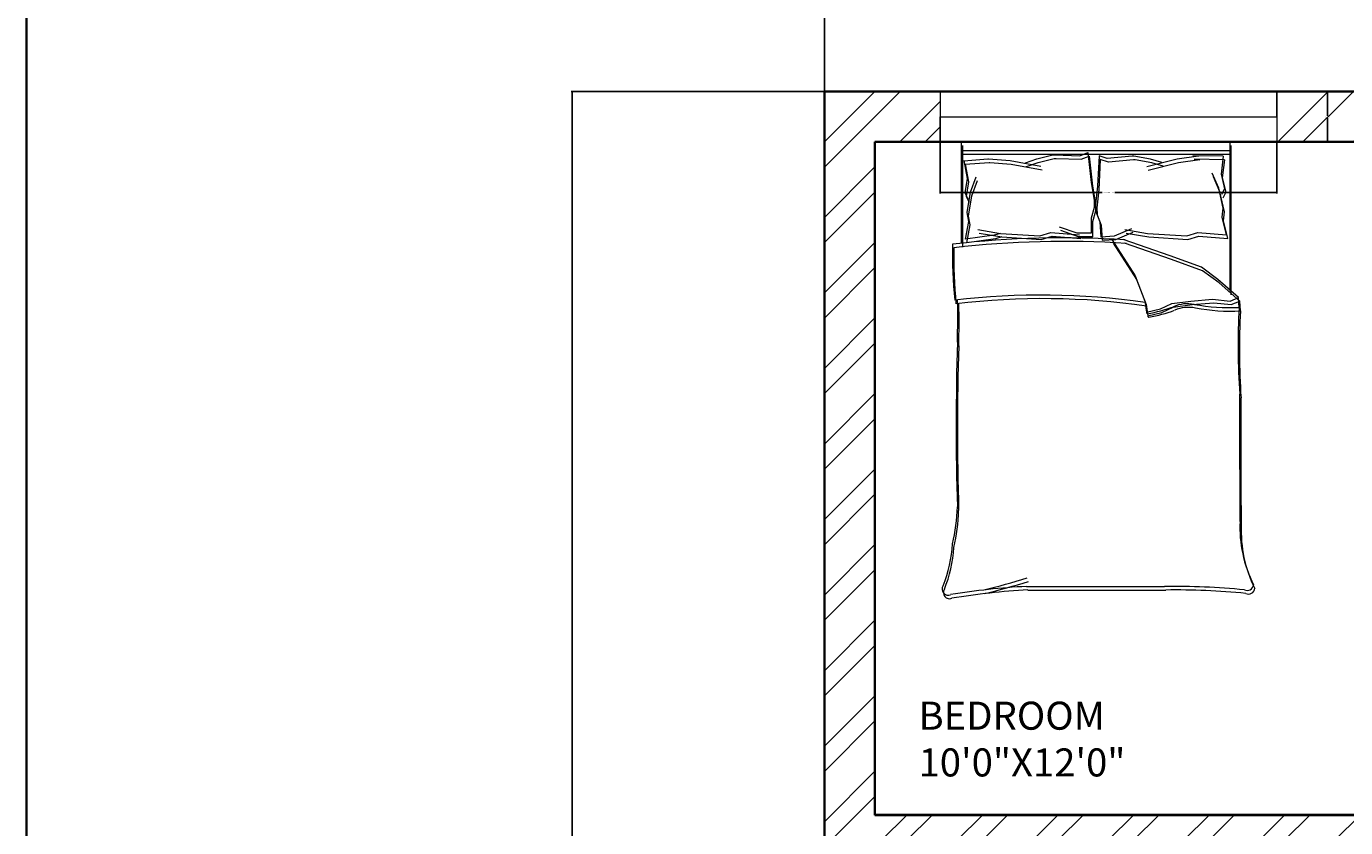
# Model space of a CAD drawing. Units: inches. Extents: x 2120 to 4013, y 1390 to 3019.
# Tile 29 of 59: x 2120 to 2356, y 2221 to 2364. Entities that reach past the tile are written whole.
import ezdxf

# ---------------------------------------------------------------- set-up
doc = ezdxf.new("R2010")
doc.units = ezdxf.units.IN
for name, color, linetype, lineweight in [('A-ANNO-DIMS', 2, 'Continuous', 18), ('A-ANNO-TTLB', 7, 'Continuous', 35), ('A-AREA-IDEN', 7, 'Continuous', 18), ('A-FURN', 8, 'Continuous', 13), ('A-GLAZ', 4, 'Continuous', 18), ('A-WALL', 7, 'Continuous', 35), ('A-WALL-PATT', 252, 'Continuous', 13)]:
    doc.layers.add(name, color=color, linetype=linetype, lineweight=lineweight)
doc.styles.get("Standard").update_dxf_attribs({"font": 'arial.ttf'})
doc.dimstyles.get("Standard").update_dxf_attribs({"dimtxt": 0.18, "dimasz": 0.18, "dimexe": 0.18, "dimexo": 0.0625, "dimgap": 0.09, "dimtad": 0, "dimtih": 1, "dimtoh": 1, "dimdec": 4, "dimzin": 0, "dimdsep": 46, "dimtxsty": 'Standard', "dimcen": 0.09, "dimadec": 0, "dimazin": 0, "dimtfac": 1, "dimtdec": 4, "dimtofl": 0, "dimtmove": 0, "dimatfit": 3, "dimfxl": 1, "dimtolj": 1, "dimtzin": 0, "dimarcsym": 0})

# ---------------------------------------------------------------- blocks, each defined once
blk = doc.blocks.new('BED-DOUBLE-PLAN')
for p, q in [((3.48, 63.34), (3.48, 81.45)), ((3.48, 81.45), (51.27, 81.45)), ((3.7, 62.7), (3.7, 80.81)), ((51.27, 81.45), (51.27, 54.84)), ((51.5, 80.81), (51.5, 54.2)), ((3.48, 79.91), (51.27, 79.91)), ((3.7, 79.27), (51.5, 79.27)), ((3.9, 78.11), (8.18, 78.44)), ((3.9, 78.13), (4.47, 74.95)), ((4.13, 77.47), (8.41, 77.8)), ((8.18, 78.44), (8.29, 78.42)), ((8.29, 78.42), (12.11, 78.13)), ((8.41, 77.8), (8.51, 77.78)), ((8.51, 77.78), (12.34, 77.49)), ((12.11, 78.13), (17.6, 77.12)), ((14.86, 77.7), (16.88, 78.42)), ((15.08, 77.06), (17.11, 77.78)), ((16.88, 78.42), (19.77, 79.14)), ((17.11, 77.78), (20, 78.5)), ((19.77, 79.14), (20.09, 79.14)), ((20, 78.5), (20.32, 78.5)), ((20.09, 79.14), (24.54, 79)), ((20.32, 78.5), (24.77, 78.36)), ((24.54, 79), (25.98, 79.58)), ((24.77, 78.36), (26.21, 78.94)), ((25.98, 79.58), (26.56, 74.23)), ((26.21, 78.94), (26.79, 73.59)), ((27.98, 78.95), (27.73, 73.58)), ((28.21, 78.32), (27.96, 72.94)), ((29.46, 78.47), (27.98, 78.95)), ((29.69, 77.83), (28.21, 78.32)), ((33.89, 78.89), (29.46, 78.47)), ((34.11, 78.25), (29.69, 77.83)), ((34.21, 78.91), (33.89, 78.89)), ((34.43, 78.27), (34.11, 78.25)), ((37.14, 78.37), (34.21, 78.91)), ((37.37, 77.73), (34.43, 78.27)), ((41.92, 78.38), (36.5, 77.02)), ((42.14, 77.74), (36.72, 76.38)), ((39.2, 77.77), (37.14, 78.37)), ((39.43, 77.13), (37.37, 77.73)), ((45.71, 78.9), (41.92, 78.38)), ((45.94, 78.26), (42.14, 77.74)), ((50.11, 78.89), (44.71, 78.99)), ((44.71, 78.99), (45.71, 78.9)), ((50.34, 78.25), (44.94, 78.35)), ((44.94, 78.35), (45.94, 78.26)), ((50.11, 78.89), (49.73, 75.68)), ((50.34, 78.25), (49.96, 75.04)), ((4.12, 77.49), (4.7, 74.31)), ((12.34, 77.49), (17.83, 76.48)), ((49.31, 73.19), (48.13, 75.87)), ((49.73, 75.68), (50.33, 73.11)), ((4.47, 74.95), (4.04, 72.35)), ((4.7, 74.31), (4.27, 71.71)), ((5.05, 72.49), (6.06, 75.24)), ((5.28, 71.85), (6.29, 74.6)), ((26.56, 74.23), (27.14, 71.05)), ((26.79, 73.59), (27.37, 70.41)), ((27.73, 73.58), (27.36, 70.37)), ((27.96, 72.94), (27.58, 69.73)), ((49.54, 72.55), (48.36, 75.23)), ((50.11, 69.62), (49.31, 73.19)), ((50.33, 73.11), (49.82, 72.06)), ((49.96, 75.04), (50.56, 72.47)), ((4.04, 72.35), (4.62, 71.33)), ((4.27, 71.71), (4.85, 70.7)), ((4.47, 68.88), (5.05, 72.49)), ((4.7, 68.24), (5.28, 71.85)), ((27.14, 71.05), (27.14, 69.74)), ((50.34, 68.98), (49.54, 72.55)), ((50.56, 72.47), (50.04, 71.42)), ((4.76, 67.29), (4.47, 68.88)), ((4.99, 66.65), (4.7, 68.24)), ((27.14, 69.74), (26.56, 67.86)), ((27.37, 69.1), (26.79, 67.23)), ((27.36, 70.37), (27.44, 69.07)), ((27.37, 70.41), (27.37, 69.1)), ((27.44, 69.07), (28.13, 67.23)), ((27.58, 69.73), (27.67, 68.43)), ((27.67, 68.43), (28.36, 66.59)), ((49.92, 68.01), (50.11, 69.62)), ((50.15, 67.37), (50.34, 68.98)), ((4.19, 64.11), (4.76, 67.29)), ((4.41, 63.47), (4.99, 66.65)), ((24.1, 65.18), (20.96, 66.27)), ((26.56, 67.86), (26.56, 65.18)), ((26.79, 67.23), (26.79, 64.54)), ((28.13, 67.23), (28.3, 64.55)), ((28.36, 66.59), (28.53, 63.91)), ((30.75, 64.71), (33.82, 65.99)), ((50.7, 64.87), (49.92, 68.01)), ((50.93, 64.23), (50.15, 67.37)), ((9.28, 64.83), (4.19, 64.11)), ((9.51, 64.19), (4.41, 63.47)), ((6.38, 65.82), (10.42, 65.15)), ((6.61, 65.18), (10.64, 64.51)), ((10.42, 65.15), (9.28, 64.83)), ((10.64, 64.51), (9.51, 64.19)), ((10.42, 65.15), (17.43, 64.72)), ((10.64, 64.51), (17.65, 64.08)), ((17.43, 64.72), (19.39, 65.28)), ((17.65, 64.08), (19.61, 64.64)), ((19.39, 65.28), (24.52, 64.87)), ((19.61, 64.64), (24.75, 64.23)), ((24.33, 64.54), (21.19, 65.63)), ((26.56, 65.18), (24.1, 65.18)), ((26.79, 64.54), (24.33, 64.54)), ((28.3, 64.55), (30.75, 64.71)), ((28.53, 63.91), (30.98, 64.07)), ((30.26, 64.06), (34.45, 57.57)), ((30.98, 64.07), (34.05, 65.35)), ((40.65, 61.13), (32.31, 64.06)), ((32.57, 65.82), (36.6, 65.15)), ((32.79, 65.18), (36.83, 64.51)), ((36.6, 65.15), (43.61, 64.72)), ((36.83, 64.51), (43.84, 64.08)), ((43.61, 64.72), (45.57, 65.28)), ((43.84, 64.08), (45.8, 64.64)), ((45.57, 65.28), (50.7, 64.87)), ((45.8, 64.64), (50.93, 64.23)), ((30.49, 63.42), (34.68, 56.93)), ((40.87, 60.49), (32.54, 63.42)), ((46.22, 59.12), (40.65, 61.13)), ((46.45, 58.48), (40.87, 60.49)), ((49.16, 56.95), (46.22, 59.12)), ((34.45, 57.57), (36.15, 53.08)), ((34.68, 56.93), (36.38, 52.44)), ((49.39, 56.31), (46.45, 58.48)), ((52.87, 53.7), (49.16, 56.95)), ((53.1, 53.06), (49.39, 56.31)), ((36.15, 53.08), (36.46, 51.07)), ((36.38, 52.44), (36.69, 50.43)), ((38.94, 51.69), (40.96, 52.62)), ((39.17, 51.05), (41.18, 51.98)), ((40.96, 52.62), (44.36, 53.08)), ((41.18, 51.98), (44.59, 52.44)), ((44.36, 53.08), (48.23, 53.39)), ((44.59, 52.44), (48.46, 52.75)), ((48.23, 53.39), (51.33, 53.08)), ((48.46, 52.75), (51.56, 52.44)), ((51.33, 53.08), (52.87, 53.7)), ((51.56, 52.44), (53.1, 53.06)), ((52.95, 51.96), (52.87, 53.7, 3.87)), ((53.18, 51.32), (53.1, 53.06, 3.87)), ((36.46, 51.07), (38.94, 51.69)), ((36.69, 50.43), (39.17, 51.05)), ((15.06, 2.2), (39.68, 2.2)), ((15.29, 1.56), (39.91, 1.56))]:
    blk.add_line(p, q)
for centre, radius, start, end in [((21.36, -100.61), 164.97, 86.0865, 96.7821), ((21.59, -101.25), 164.97, 86.0865, 96.7821), ((85.16, 61.35), 83.31, 178.7218, 185.604), ((85.39, 60.71), 83.31, 178.7218, 185.604), ((17.76, -74.87), 129.02, 81.7845, 96.9006), ((17.99, -75.51), 129.02, 81.7845, 96.9006), ((-167.31, 50.27), 170.11, 358.4762, 1.0082), ((-167.08, 49.63), 170.11, 358.4762, 1.0082), ((31.16, 79.96), 29.65, 280.6617, 289.8806), ((43.74, 46.38), 6.22, 78.6608, 113.7384), ((43.97, 45.74), 6.22, 78.6608, 113.7384), ((51.33, 88.1), 36.18, 259.8763, 272.5657), ((51.56, 87.46), 36.18, 259.8763, 272.5657), ((182.27, 45.13), 129.5, 176.9791, 183.8365), ((36.64, 51.01), 0.185, 160.2464, 271.1377), ((36.87, 50.37), 0.185, 160.2464, 271.1377), ((31.38, 79.32), 29.65, 280.6617, 289.8806), ((182.5, 44.49), 129.5, 176.9791, 183.8365), ((484.82, 30.83), 482.31, 178.2277, 181.7185), ((485.05, 30.19), 482.31, 178.2277, 181.7185), ((-4508.74, 13.62), 4561.86, 0.00217, 0.28689), ((-4508.51, 12.99), 4561.86, 0.00217, 0.28689), ((-26.9, 16.93), 29.63, 346.0648, 358.9113), ((-26.67, 16.29), 29.63, 346.0648, 358.9113), ((76.16, 12.78), 23.07, 177.4714, 206.4681), ((76.39, 12.14), 23.07, 177.4714, 206.4681), ((-21.66, 11.17), 23.56, 337.9751, 356.652), ((-21.43, 10.53), 23.56, 337.9751, 356.652), ((-17.22, 105.16), 106.46, 283.3832, 287.7053), ((-16.99, 104.52), 106.46, 283.3832, 287.7053), ((54.41, 2.58), 1.1, 242.6588, 356.02), ((1.09, 1.73), 1.09, 146.1736, 293.4781), ((1.32, 1.09), 1.09, 146.1736, 293.4781), ((21.43, -119.39), 121.76, 92.9958, 99.4091), ((21.66, -120.03), 121.76, 92.9958, 99.4091), ((41.15, -130.83), 133.04, 84.4998, 90.6351), ((41.38, -131.47), 133.04, 84.4998, 90.6351), ((54.64, 1.94), 1.1, 242.6588, 356.02)]:
    blk.add_arc(centre, radius, start, end)
blk = doc.blocks.new('WIN-PLAN-60IN')
for p, q in [((0, 9), (0, 0)), ((60, 4.5), (60, 9)), ((60, 9), (60, 0)), ((0, 0), (0, 4.5)), ((0, 4.5), (60, 4.5))]:
    blk.add_line(p, q)
blk = doc.blocks.new('*D171')
at = {"layer": 'A-ANNO-DIMS', "color": 0, "lineweight": -2, "transparency": 16777216}
for p, q in [((2283.38, 2343.47), (2283.38, 2334.35)), ((2343.38, 2343.47), (2343.38, 2334.35)), ((2283.56, 2334.53), (2312.26, 2334.53)), ((2343.2, 2334.53), (2314.5, 2334.53))]:
    blk.add_line(p, q, dxfattribs=at)
at = {"layer": 'A-ANNO-DIMS', "color": 0, "transparency": 16777216}
for points in [[(2283.56, 2334.56), (2283.56, 2334.5), (2283.38, 2334.53)], [(2343.2, 2334.56), (2343.2, 2334.5), (2343.38, 2334.53)]]:
    blk.add_solid(points, dxfattribs=at)
at = {"layer": 'Defpoints', "color": 0, "transparency": 16777216}
for p in [(2283.38, 2343.53), (2343.38, 2343.53), (2343.38, 2334.53)]:
    blk.add_point(p, dxfattribs=at)
at = {"layer": 'A-ANNO-DIMS', "color": 0, "transparency": 16777216, "insert": (2313.38, 2334.53), "char_height": 0.18, "attachment_point": 5}
blk.add_mtext('\\A1;WINDOW 60 TYP.', dxfattribs=at)
blk = doc.blocks.new('*D172')
at = {"layer": 'A-ANNO-DIMS', "color": 0, "lineweight": -2, "transparency": 16777216}
for p, q in [((2343.44, 2352.53), (2352.56, 2352.53)), ((2352.38, 2352.35), (2352.38, 2348.21)), ((2352.38, 2343.71), (2352.38, 2347.85)), ((2343.44, 2343.53), (2352.56, 2343.53))]:
    blk.add_line(p, q, dxfattribs=at)
at = {"layer": 'A-ANNO-DIMS', "color": 0, "transparency": 16777216}
for points in [[(2352.35, 2352.35), (2352.41, 2352.35), (2352.38, 2352.53)], [(2352.35, 2343.71), (2352.41, 2343.71), (2352.38, 2343.53)]]:
    blk.add_solid(points, dxfattribs=at)
at = {"layer": 'Defpoints', "color": 0, "transparency": 16777216}
for p in [(2343.38, 2352.53), (2352.38, 2352.53), (2343.38, 2343.53)]:
    blk.add_point(p, dxfattribs=at)
at = {"layer": 'A-ANNO-DIMS', "color": 0, "transparency": 16777216, "insert": (2352.38, 2348.03), "char_height": 0.18, "attachment_point": 5}
blk.add_mtext('\\A1;9 TYP.', dxfattribs=at)
blk = doc.blocks.new('*D211')
at = {"layer": 'A-ANNO-DIMS', "color": 0, "lineweight": -2, "transparency": 16777216}
for p, q in [((2262.73, 2352.59), (2262.73, 2397.71)), ((2262.91, 2397.53), (2635.95, 2397.53)), ((3009.55, 2397.53), (2636.52, 2397.53)), ((3009.73, 2352.59), (3009.73, 2397.71))]:
    blk.add_line(p, q, dxfattribs=at)
at = {"layer": 'A-ANNO-DIMS', "color": 0, "transparency": 16777216}
for points in [[(2262.91, 2397.56), (2262.91, 2397.5), (2262.73, 2397.53)], [(3009.55, 2397.56), (3009.55, 2397.5), (3009.73, 2397.53)]]:
    blk.add_solid(points, dxfattribs=at)
at = {"layer": 'Defpoints', "color": 0, "transparency": 16777216}
for p in [(3009.73, 2397.53), (2262.73, 2352.53), (3009.73, 2352.53)]:
    blk.add_point(p, dxfattribs=at)
at = {"layer": 'A-ANNO-DIMS', "color": 0, "transparency": 16777216, "insert": (2636.23, 2397.53), "char_height": 0.18, "attachment_point": 5}
blk.add_mtext('\\A1;747', dxfattribs=at)
blk = doc.blocks.new('*D215')
at = {"layer": 'A-ANNO-DIMS', "color": 0, "lineweight": -2, "transparency": 16777216}
for p, q in [((2262.67, 2352.53), (2217.55, 2352.53)), ((2217.73, 2352.35), (2217.73, 2213.96)), ((2217.73, 2075.21), (2217.73, 2213.6)), ((2271.67, 2075.03), (2217.55, 2075.03))]:
    blk.add_line(p, q, dxfattribs=at)
at = {"layer": 'A-ANNO-DIMS', "color": 0, "transparency": 16777216}
for points in [[(2217.7, 2352.35), (2217.76, 2352.35), (2217.73, 2352.53)], [(2217.7, 2075.21), (2217.76, 2075.21), (2217.73, 2075.03)]]:
    blk.add_solid(points, dxfattribs=at)
at = {"layer": 'Defpoints', "color": 0, "transparency": 16777216}
for p in [(2217.73, 2352.53), (2262.73, 2352.53), (2271.73, 2075.03)]:
    blk.add_point(p, dxfattribs=at)
at = {"layer": 'A-ANNO-DIMS', "color": 0, "transparency": 16777216, "insert": (2217.73, 2213.78), "char_height": 0.18, "attachment_point": 5}
blk.add_mtext('\\A1;277.5', dxfattribs=at)

msp = doc.modelspace()

# ---------------------------------------------------------------- hatches: boundary and pattern name
at = {"layer": 'A-WALL-PATT'}
h = msp.add_hatch(dxfattribs=at)
h.set_pattern_fill('ANSI32', color=256)
h.paths.add_polyline_path([(2271.7331, 2343.531), (2283.3788, 2343.531), (2283.3788, 2348.031), (2283.3788, 2352.5306), (2262.7331, 2352.5306), (2262.7331, 2182.638), (2267.2331, 2182.638), (2271.7331, 2182.638), (2271.7331, 2219.031), (2391.7331, 2219.031), (2391.7331, 2214.189), (2393.9831, 2214.189), (2396.2331, 2214.189), (2396.2331, 2219.031), (2420.2331, 2219.031), (2420.2331, 2225.7535), (2417.2197, 2225.7535), (2415.7331, 2225.7535), (2415.7331, 2223.5306), (2271.7331, 2223.5306)])
h.paths.add_polyline_path([(2380.0942, 2352.5306), (2343.3788, 2352.5306), (2343.3788, 2343.531), (2363.2331, 2343.531), (2363.2331, 2288.8489), (2365.4831, 2288.8489), (2367.7331, 2288.8489), (2367.7331, 2343.531), (2380.0942, 2343.531)], flags=17)
h.paths.add_polyline_path([(2432.4339, 2352.5306), (2404.0943, 2352.5306), (2404.0943, 2343.531), (2415.7331, 2343.531), (2415.7331, 2264.0306), (2367.7331, 2264.0306), (2367.7331, 2266.4872), (2363.2331, 2266.4872), (2363.2331, 2259.531), (2367.7331, 2259.531), (2415.7331, 2259.531), (2415.7331, 2255.0658), (2420.2331, 2255.0658), (2420.2331, 2259.531), (2424.5717, 2259.531), (2424.5717, 2261.781), (2424.5717, 2264.0306), (2420.2331, 2264.0306), (2420.2331, 2343.531), (2432.4339, 2343.531)])
h.paths.add_polyline_path([(2508.9115, 2352.5306), (2456.4339, 2352.5306), (2456.4339, 2343.531), (2468.2331, 2343.531), (2468.2331, 2264.0306), (2448.0487, 2264.0306), (2448.0487, 2259.531), (2468.2331, 2259.531), (2468.2331, 2255.5496), (2472.7331, 2255.5496), (2472.7331, 2343.531), (2508.9115, 2343.531)])
h.paths.add_polyline_path([(2637.7331, 2352.5306), (2544.9116, 2352.5306), (2544.9116, 2343.531), (2589.7331, 2343.531), (2633.2331, 2343.531), (2637.7331, 2343.531)])
h.paths.add_polyline_path([(2594.2331, 2343.5306), (2589.7331, 2343.5306), (2589.7331, 2259.5306), (2589.7331, 2252.4915), (2591.9831, 2252.4915), (2594.2331, 2252.4915)])
h.paths.add_polyline_path([(2637.7331, 2223.5306), (2594.2331, 2223.5306), (2594.2331, 2230.1988), (2591.9831, 2230.1988), (2589.7331, 2230.1988), (2589.7331, 2223.5306), (2472.7331, 2223.5306), (2468.2331, 2223.5306), (2468.2331, 2219.031), (2628.7331, 2219.031), (2628.7331, 2138.031), (2637.7331, 2138.031)])
h.paths.add_polyline_path([(3822.6535, 2458.4402), (3874.9468, 2458.4402), (3874.9468, 2476.9866), (3822.6535, 2476.9866)], flags=9)
h.paths.add_polyline_path([(3834.6921, 2781.8174), (3935.9206, 2781.8174), (3935.9206, 2800.3638), (3834.6921, 2800.3638)], flags=9)
h.paths.add_polyline_path([(3832.2843, 2837.9683), (3884.5776, 2837.9683), (3884.5776, 2856.5146), (3832.2843, 2856.5146)], flags=9)
h.paths.add_polyline_path([(3830.9388, 2861.4782), (3956.8958, 2861.4782), (3956.8958, 2880.0245), (3830.9388, 2880.0245)], flags=9)
h.paths.add_polyline_path([(3870.6966, 2352.5752), (3887.9272, 2352.5752), (3887.9272, 2377.3037), (3870.6966, 2377.3037)], flags=9)
h.paths.add_polyline_path([(3289.2701, 2413.161), (3435.2223, 2413.161), (3435.2223, 2450.2538), (3289.2701, 2450.2538)], flags=9)
h.paths.add_polyline_path([(2487.6944, 2414.3601), (2637.8335, 2414.3601), (2637.8335, 2451.4528), (2487.6944, 2451.4528)], flags=9)
h.paths.add_polyline_path([(2567.3724, 1457.9199), (2815.296, 1457.9199), (2815.296, 1495.0127), (2567.3724, 1495.0127)], flags=9)
h.paths.add_polyline_path([(2655.3825, 2093.2363), (2685.9555, 2093.2363), (2685.9555, 2111.8937), (2655.3825, 2111.8937)], flags=9)
h.paths.add_polyline_path([(2543.9218, 1550.6671), (2587.8406, 1550.6671), (2587.8406, 1569.3244), (2543.9218, 1569.3244)], flags=9)
h.paths.add_polyline_path([(2905.1384, 1543.8113), (2949.0572, 1543.8113), (2949.0572, 1562.4686), (2905.1384, 1562.4686)], flags=9)
h.paths.add_polyline_path([(2736.4118, 1702.4736), (2784.2153, 1702.4736), (2784.2153, 1721.1309), (2736.4118, 1721.1309)], flags=9)
h.paths.add_polyline_path([(2912.8666, 1710.4168), (2951.707, 1710.4168), (2951.707, 1729.0741), (2912.8666, 1729.0741)], flags=9)
h.paths.add_polyline_path([(2923.5785, 1763.5038), (2959.7279, 1763.5038), (2959.7279, 1782.1611), (2923.5785, 1782.1611)], flags=9)
h.paths.add_polyline_path([(2925.2114, 1809.6137), (2967.1861, 1809.6137), (2967.1861, 1828.271), (2925.2114, 1828.271)], flags=9)
h.paths.add_polyline_path([(2996.2711, 1878.9003), (2996.2711, 1913.109), (2977.6138, 1913.109), (2977.6138, 1878.9003)], flags=9)
h.paths.add_polyline_path([(2883.0859, 1895.7192), (2927.1855, 1895.7192), (2927.1855, 1914.3766), (2883.0859, 1914.3766)], flags=9)
h.paths.add_polyline_path([(2787.3924, 1810.8013), (2841.0213, 1810.8013), (2841.0213, 1829.4587), (2787.3924, 1829.4587)], flags=9)
h.paths.add_polyline_path([(2775.6399, 2101.7395), (2829.2689, 2101.7395), (2829.2689, 2120.3968), (2775.6399, 2120.3968)], flags=9)
h.paths.add_polyline_path([(2913.0263, 2075.817), (2951.8667, 2075.817), (2951.8667, 2094.4744), (2913.0263, 2094.4744)], flags=9)
h.paths.add_polyline_path([(2929.966, 2133.3669), (2966.1154, 2133.3669), (2966.1154, 2152.0243), (2929.966, 2152.0243)], flags=9)
h.paths.add_polyline_path([(2932.7502, 2182.6088), (2968.8996, 2182.6088), (2968.8996, 2201.2662), (2932.7502, 2201.2662)], flags=9)
h.paths.add_polyline_path([(2996.0681, 2266.3173), (2996.0681, 2300.5261), (2977.4108, 2300.5261), (2977.4108, 2266.3173)], flags=9)
h.paths.add_polyline_path([(2885.1039, 2279.2186), (2929.2035, 2279.2186), (2929.2035, 2297.8759), (2885.1039, 2297.8759)], flags=9)
h.paths.add_polyline_path([(2735.7042, 2218.3197), (2783.5078, 2218.3197), (2783.5078, 2236.9771), (2735.7042, 2236.9771)], flags=9)
h.paths.add_polyline_path([(2635.6049, 2044.0085), (2648.9678, 2044.0085), (2648.9678, 2054.312), (2635.6049, 2054.312)], flags=9)
h.paths.add_polyline_path([(2714.0148, 1923.0473), (2727.3777, 1923.0473), (2727.3777, 1933.3508), (2714.0148, 1933.3508)], flags=9)
h.paths.add_polyline_path([(2709.0345, 1988.1628), (2722.3974, 1988.1628), (2722.3974, 1998.4663), (2709.0345, 1998.4663)], flags=9)
h.paths.add_polyline_path([(2592.8935, 1962.1763), (2606.2564, 1962.1763), (2606.2564, 1972.4799), (2592.8935, 1972.4799)], flags=9)
h.paths.add_polyline_path([(2618.3996, 1985.9724), (2644.1942, 1985.9724), (2644.1942, 1996.2759), (2618.3996, 1996.2759)], flags=9)
h.paths.add_polyline_path([(2601.279, 1920.5869), (2614.6419, 1920.5869), (2614.6419, 1930.8904), (2601.279, 1930.8904)], flags=9)
h.paths.add_polyline_path([(2692.3278, 1932.7645), (2704.5311, 1932.7645), (2704.5311, 1943.0681), (2692.3278, 1943.0681)], flags=9)
h.paths.add_polyline_path([(2311.122, 1672.7318), (2355.0408, 1672.7318), (2355.0408, 1691.3892), (2311.122, 1691.3892)], flags=9)
h.paths.add_polyline_path([(2456.2551, 1632.3198), (2492.4796, 1632.3198), (2492.4796, 1650.9772), (2456.2551, 1650.9772)], flags=9)
h.paths.add_polyline_path([(2401.0766, 1631.4793), (2437.301, 1631.4793), (2437.301, 1650.1367), (2401.0766, 1650.1367)], flags=9)
h.paths.add_polyline_path([(2546.7054, 1700.9235), (2594.509, 1700.9235), (2594.509, 1719.5809), (2546.7054, 1719.5809)], flags=9)
h.paths.add_polyline_path([(2445.4866, 1766.9937), (2497.5261, 1766.9937), (2497.5261, 1785.651), (2445.4866, 1785.651)], flags=9)
h.paths.add_polyline_path([(2287.9992, 1739.7675), (2326.8396, 1739.7675), (2326.8396, 1758.4248), (2287.9992, 1758.4248)], flags=9)
h.paths.add_polyline_path([(2458.5279, 1924.7607), (2510.5675, 1924.7607), (2510.5675, 1943.4181), (2458.5279, 1943.4181)], flags=9)
h.paths.add_polyline_path([(2309.2811, 1902.7642), (2345.4305, 1902.7642), (2345.4305, 1921.4215), (2309.2811, 1921.4215)], flags=9)
h.paths.add_polyline_path([(2490.7554, 2018.9392), (2530.7896, 2018.9392), (2530.7896, 2037.5965), (2490.7554, 2037.5965)], flags=9)
h.paths.add_polyline_path([(2402.143, 2024.7393), (2438.5414, 2024.7393), (2438.5414, 2043.3966), (2402.143, 2043.3966)], flags=9)
h.paths.add_polyline_path([(2287.856, 1931.7926), (2326.6964, 1931.7926), (2326.6964, 1950.4499), (2287.856, 1950.4499)], flags=9)
h.paths.add_polyline_path([(2281.7979, 2193.5771), (2320.6383, 2193.5771), (2320.6383, 2212.2344), (2281.7979, 2212.2344)], flags=25)
h.paths.add_polyline_path([(2484.0754, 2093.892), (2536.115, 2093.892), (2536.115, 2112.5494), (2484.0754, 2112.5494)], flags=9)
h.paths.add_polyline_path([(2624.7948, 2281.8639), (2624.7948, 2311.4137), (2606.1375, 2311.4137), (2606.1375, 2281.8639)], flags=9)
h.paths.add_polyline_path([(2507.5036, 2290.3639), (2541.934, 2290.3639), (2541.934, 2309.0212), (2507.5036, 2309.0212)], flags=9)
h.paths.add_polyline_path([(2423.1076, 2285.2202), (2459.332, 2285.2202), (2459.332, 2303.8776), (2423.1076, 2303.8776)], flags=9)
h.paths.add_polyline_path([(2374.5467, 2289.6272), (2410.7711, 2289.6272), (2410.7711, 2308.2846), (2374.5467, 2308.2846)], flags=25)
h.paths.add_polyline_path([(2277.4907, 2227.5651), (2316.3311, 2227.5651), (2316.3311, 2246.2224), (2277.4907, 2246.2224)], flags=25)
h.paths.add_polyline_path([(2655.3825, 2093.2367), (2685.9555, 2093.2367), (2685.9555, 2111.894), (2655.3825, 2111.894)], flags=9)
h.paths.add_polyline_path([(2543.9217, 1550.6674), (2587.8406, 1550.6674), (2587.8406, 1569.3247), (2543.9217, 1569.3247)], flags=9)
h.paths.add_polyline_path([(2905.1384, 1543.8116), (2949.0572, 1543.8116), (2949.0572, 1562.4689), (2905.1384, 1562.4689)], flags=9)
h.paths.add_polyline_path([(2736.4118, 1702.4739), (2784.2153, 1702.4739), (2784.2153, 1721.1312), (2736.4118, 1721.1312)], flags=9)
h.paths.add_polyline_path([(2912.8666, 1710.4171), (2951.707, 1710.4171), (2951.707, 1729.0744), (2912.8666, 1729.0744)], flags=9)
h.paths.add_polyline_path([(2923.5785, 1763.5041), (2959.7279, 1763.5041), (2959.7279, 1782.1614), (2923.5785, 1782.1614)], flags=9)
h.paths.add_polyline_path([(2925.2114, 1809.614), (2967.1861, 1809.614), (2967.1861, 1828.2713), (2925.2114, 1828.2713)], flags=9)
h.paths.add_polyline_path([(2996.2711, 1878.9006), (2996.2711, 1913.1094), (2977.6137, 1913.1094), (2977.6137, 1878.9006)], flags=9)
h.paths.add_polyline_path([(2883.0859, 1895.7195), (2927.1855, 1895.7195), (2927.1855, 1914.3769), (2883.0859, 1914.3769)], flags=9)
h.paths.add_polyline_path([(2787.3924, 1810.8016), (2841.0213, 1810.8016), (2841.0213, 1829.459), (2787.3924, 1829.459)], flags=9)
h.paths.add_polyline_path([(2775.6399, 2101.7398), (2829.2688, 2101.7398), (2829.2688, 2120.3971), (2775.6399, 2120.3971)], flags=9)
h.paths.add_polyline_path([(2913.0263, 2075.8173), (2951.8667, 2075.8173), (2951.8667, 2094.4747), (2913.0263, 2094.4747)], flags=9)
h.paths.add_polyline_path([(2929.966, 2133.3672), (2966.1154, 2133.3672), (2966.1154, 2152.0246), (2929.966, 2152.0246)], flags=9)
h.paths.add_polyline_path([(2932.7502, 2182.6091), (2968.8996, 2182.6091), (2968.8996, 2201.2665), (2932.7502, 2201.2665)], flags=9)
h.paths.add_polyline_path([(2996.0681, 2266.3176), (2996.0681, 2300.5264), (2977.4108, 2300.5264), (2977.4108, 2266.3176)], flags=9)
h.paths.add_polyline_path([(2885.1039, 2279.2189), (2929.2035, 2279.2189), (2929.2035, 2297.8762), (2885.1039, 2297.8762)], flags=9)
h.paths.add_polyline_path([(2735.7042, 2218.32), (2783.5078, 2218.32), (2783.5078, 2236.9774), (2735.7042, 2236.9774)], flags=9)
h.paths.add_polyline_path([(2635.6048, 2044.0088), (2648.9677, 2044.0088), (2648.9677, 2054.3123), (2635.6048, 2054.3123)], flags=9)
h.paths.add_polyline_path([(2714.0148, 1923.0476), (2727.3777, 1923.0476), (2727.3777, 1933.3511), (2714.0148, 1933.3511)], flags=9)
h.paths.add_polyline_path([(2709.0345, 1988.1631), (2722.3974, 1988.1631), (2722.3974, 1998.4666), (2709.0345, 1998.4666)], flags=9)
h.paths.add_polyline_path([(2592.8935, 1962.1766), (2606.2564, 1962.1766), (2606.2564, 1972.4802), (2592.8935, 1972.4802)], flags=9)
h.paths.add_polyline_path([(2618.3995, 1985.9727), (2644.1942, 1985.9727), (2644.1942, 1996.2762), (2618.3995, 1996.2762)], flags=9)
h.paths.add_polyline_path([(2601.279, 1920.5872), (2614.6419, 1920.5872), (2614.6419, 1930.8908), (2601.279, 1930.8908)], flags=9)
h.paths.add_polyline_path([(2692.3278, 1932.7648), (2704.5311, 1932.7648), (2704.5311, 1943.0684), (2692.3278, 1943.0684)], flags=9)
h.paths.add_polyline_path([(2311.122, 1672.7321), (2355.0408, 1672.7321), (2355.0408, 1691.3895), (2311.122, 1691.3895)], flags=9)
h.paths.add_polyline_path([(2456.2551, 1632.3201), (2492.4795, 1632.3201), (2492.4795, 1650.9775), (2456.2551, 1650.9775)], flags=9)
h.paths.add_polyline_path([(2401.0766, 1631.4796), (2437.301, 1631.4796), (2437.301, 1650.137), (2401.0766, 1650.137)], flags=9)
h.paths.add_polyline_path([(2546.7054, 1700.9238), (2594.509, 1700.9238), (2594.509, 1719.5812), (2546.7054, 1719.5812)], flags=9)
h.paths.add_polyline_path([(2445.4866, 1766.994), (2497.5261, 1766.994), (2497.5261, 1785.6513), (2445.4866, 1785.6513)], flags=9)
h.paths.add_polyline_path([(2287.9992, 1739.7678), (2326.8396, 1739.7678), (2326.8396, 1758.4251), (2287.9992, 1758.4251)], flags=9)
h.paths.add_polyline_path([(2458.5279, 1924.7611), (2510.5675, 1924.7611), (2510.5675, 1943.4184), (2458.5279, 1943.4184)], flags=9)
h.paths.add_polyline_path([(2309.2811, 1902.7645), (2345.4305, 1902.7645), (2345.4305, 1921.4218), (2309.2811, 1921.4218)], flags=9)
h.paths.add_polyline_path([(2490.7554, 2018.9395), (2530.7895, 2018.9395), (2530.7895, 2037.5968), (2490.7554, 2037.5968)], flags=9)
h.paths.add_polyline_path([(2402.143, 2024.7396), (2438.5413, 2024.7396), (2438.5413, 2043.3969), (2402.143, 2043.3969)], flags=9)
h.paths.add_polyline_path([(2287.856, 1931.7929), (2326.6964, 1931.7929), (2326.6964, 1950.4502), (2287.856, 1950.4502)], flags=9)
h.paths.add_polyline_path([(2281.7979, 2193.5774), (2320.6383, 2193.5774), (2320.6383, 2212.2347), (2281.7979, 2212.2347)], flags=25)
h.paths.add_polyline_path([(2484.0754, 2093.8924), (2536.115, 2093.8924), (2536.115, 2112.5497), (2484.0754, 2112.5497)], flags=9)
h.paths.add_polyline_path([(2624.7948, 2281.8642), (2624.7948, 2311.414), (2606.1374, 2311.414), (2606.1374, 2281.8642)], flags=9)
h.paths.add_polyline_path([(2507.5035, 2290.3642), (2541.934, 2290.3642), (2541.934, 2309.0215), (2507.5035, 2309.0215)], flags=9)
h.paths.add_polyline_path([(2423.1075, 2285.2205), (2459.332, 2285.2205), (2459.332, 2303.8779), (2423.1075, 2303.8779)], flags=9)
h.paths.add_polyline_path([(2374.5467, 2289.6275), (2410.7711, 2289.6275), (2410.7711, 2308.2849), (2374.5467, 2308.2849)], flags=25)
h.paths.add_polyline_path([(2277.4907, 2227.5654), (2316.3311, 2227.5654), (2316.3311, 2246.2227), (2277.4907, 2246.2227)], flags=25)
h = msp.add_hatch(dxfattribs=at)
h.set_pattern_fill('ANSI32', color=256)
h.paths.add_polyline_path([(2271.7331, 1980.389), (2262.7331, 1980.389), (2262.7331, 1912.8434), (2267.2331, 1912.8434), (2271.7331, 1912.8434), (2271.7331, 1922.531), (2351.2331, 1922.531), (2351.2331, 1901.4728), (2355.7331, 1901.4728), (2355.7331, 1922.531), (2357.9815, 1922.531), (2357.9815, 1926.5306), (2271.7331, 1926.5306)])
h.paths.add_polyline_path([(2589.2331, 1949.1622), (2584.7331, 1949.1622), (2580.2331, 1949.1622), (2580.2331, 1874.5306), (2355.7331, 1874.5306), (2355.7331, 1880.1922), (2351.2331, 1880.1922), (2351.2331, 1874.5306), (2271.7331, 1874.5306), (2271.7331, 1888.8431), (2262.7331, 1888.8431), (2262.7331, 1842.2909), (2267.2331, 1842.2909), (2271.7331, 1842.2909), (2271.7331, 1865.531), (2415.7331, 1865.531), (2415.7331, 1779.7286), (2420.2331, 1779.7286), (2420.2331, 1865.531), (2589.2331, 1865.531)])
h.paths.add_polyline_path([(2271.7331, 1782.2906), (2262.7331, 1782.2906), (2262.7331, 1711.4639), (2267.2331, 1711.4639), (2271.7331, 1711.4639), (2271.7331, 1738.031), (2420.2331, 1738.031), (2420.2331, 1742.531), (2420.2331, 1747.3376), (2417.9831, 1747.3376), (2415.7331, 1747.3376), (2415.7331, 1742.5306), (2271.7331, 1742.5306)])
h.paths.add_polyline_path([(2271.7331, 1627.031), (2362.3957, 1627.031), (2362.3957, 1629.281), (2362.3957, 1631.5306), (2271.7331, 1631.5306), (2271.7331, 1675.4636), (2262.7331, 1675.4636), (2262.7331, 1581.531), (2405.3032, 1581.531), (2405.3032, 1586.031), (2405.3032, 1590.5306), (2396.2331, 1590.5306), (2396.2331, 1691.4513), (2418.7206, 1691.4513), (2418.7206, 1695.951), (2396.2331, 1695.951), (2391.7331, 1695.951), (2391.7331, 1631.5306), (2386.7425, 1631.5306), (2386.7425, 1629.2806), (2386.7425, 1627.031), (2391.7331, 1627.031), (2391.7331, 1586.1709), (2271.7331, 1586.1709)])
h.paths.add_polyline_path([(2459.6703, 1590.5306), (2429.3032, 1590.5306), (2429.3032, 1581.531), (2459.6703, 1581.531), (2459.6703, 1586.031)])
h.paths.add_polyline_path([(2501.2331, 1590.531), (2501.2331, 1665.0195), (2498.9831, 1665.0195), (2496.7331, 1665.0195), (2496.7331, 1590.5306), (2483.8201, 1590.5306), (2483.8201, 1590.1579), (2483.6704, 1590.1579), (2483.6704, 1581.531), (2505.0196, 1581.531), (2505.0196, 1583.781), (2505.0196, 1586.0306), (2501.2331, 1586.0306)])
h.paths.add_polyline_path([(2544.1361, 1583.781), (2544.1361, 1586.0306), (2527.1368, 1586.0306), (2527.1368, 1583.7806), (2527.1368, 1581.531), (2544.1361, 1581.531)])
h.paths.add_polyline_path([(3822.6535, 2458.4402), (3874.9468, 2458.4402), (3874.9468, 2476.9866), (3822.6535, 2476.9866)], flags=9)
h.paths.add_polyline_path([(3834.6921, 2781.8174), (3935.9206, 2781.8174), (3935.9206, 2800.3638), (3834.6921, 2800.3638)], flags=9)
h.paths.add_polyline_path([(3832.2843, 2837.9683), (3884.5776, 2837.9683), (3884.5776, 2856.5146), (3832.2843, 2856.5146)], flags=9)
h.paths.add_polyline_path([(3830.9388, 2861.4782), (3956.8958, 2861.4782), (3956.8958, 2880.0245), (3830.9388, 2880.0245)], flags=9)
h.paths.add_polyline_path([(3870.6966, 2352.5752), (3887.9272, 2352.5752), (3887.9272, 2377.3037), (3870.6966, 2377.3037)], flags=9)
h.paths.add_polyline_path([(3289.2701, 2413.161), (3435.2223, 2413.161), (3435.2223, 2450.2538), (3289.2701, 2450.2538)], flags=9)
h.paths.add_polyline_path([(2487.6944, 2414.3601), (2637.8335, 2414.3601), (2637.8335, 2451.4528), (2487.6944, 2451.4528)], flags=9)
h.paths.add_polyline_path([(2567.3724, 1457.9199), (2815.296, 1457.9199), (2815.296, 1495.0127), (2567.3724, 1495.0127)], flags=9)
h.paths.add_polyline_path([(2655.3825, 2093.2363), (2685.9555, 2093.2363), (2685.9555, 2111.8937), (2655.3825, 2111.8937)], flags=9)
h.paths.add_polyline_path([(2543.9218, 1550.6671), (2587.8406, 1550.6671), (2587.8406, 1569.3244), (2543.9218, 1569.3244)], flags=9)
h.paths.add_polyline_path([(2905.1384, 1543.8113), (2949.0572, 1543.8113), (2949.0572, 1562.4686), (2905.1384, 1562.4686)], flags=9)
h.paths.add_polyline_path([(2736.4118, 1702.4736), (2784.2153, 1702.4736), (2784.2153, 1721.1309), (2736.4118, 1721.1309)], flags=9)
h.paths.add_polyline_path([(2912.8666, 1710.4168), (2951.707, 1710.4168), (2951.707, 1729.0741), (2912.8666, 1729.0741)], flags=9)
h.paths.add_polyline_path([(2923.5785, 1763.5038), (2959.7279, 1763.5038), (2959.7279, 1782.1611), (2923.5785, 1782.1611)], flags=9)
h.paths.add_polyline_path([(2925.2114, 1809.6137), (2967.1861, 1809.6137), (2967.1861, 1828.271), (2925.2114, 1828.271)], flags=9)
h.paths.add_polyline_path([(2996.2711, 1878.9003), (2996.2711, 1913.109), (2977.6138, 1913.109), (2977.6138, 1878.9003)], flags=9)
h.paths.add_polyline_path([(2883.0859, 1895.7192), (2927.1855, 1895.7192), (2927.1855, 1914.3766), (2883.0859, 1914.3766)], flags=9)
h.paths.add_polyline_path([(2787.3924, 1810.8013), (2841.0213, 1810.8013), (2841.0213, 1829.4587), (2787.3924, 1829.4587)], flags=9)
h.paths.add_polyline_path([(2775.6399, 2101.7395), (2829.2689, 2101.7395), (2829.2689, 2120.3968), (2775.6399, 2120.3968)], flags=9)
h.paths.add_polyline_path([(2913.0263, 2075.817), (2951.8667, 2075.817), (2951.8667, 2094.4744), (2913.0263, 2094.4744)], flags=9)
h.paths.add_polyline_path([(2929.966, 2133.3669), (2966.1154, 2133.3669), (2966.1154, 2152.0243), (2929.966, 2152.0243)], flags=9)
h.paths.add_polyline_path([(2932.7502, 2182.6088), (2968.8996, 2182.6088), (2968.8996, 2201.2662), (2932.7502, 2201.2662)], flags=9)
h.paths.add_polyline_path([(2996.0681, 2266.3173), (2996.0681, 2300.5261), (2977.4108, 2300.5261), (2977.4108, 2266.3173)], flags=9)
h.paths.add_polyline_path([(2885.1039, 2279.2186), (2929.2035, 2279.2186), (2929.2035, 2297.8759), (2885.1039, 2297.8759)], flags=9)
h.paths.add_polyline_path([(2735.7042, 2218.3197), (2783.5078, 2218.3197), (2783.5078, 2236.9771), (2735.7042, 2236.9771)], flags=9)
h.paths.add_polyline_path([(2635.6049, 2044.0085), (2648.9678, 2044.0085), (2648.9678, 2054.312), (2635.6049, 2054.312)], flags=9)
h.paths.add_polyline_path([(2714.0148, 1923.0473), (2727.3777, 1923.0473), (2727.3777, 1933.3508), (2714.0148, 1933.3508)], flags=9)
h.paths.add_polyline_path([(2709.0345, 1988.1628), (2722.3974, 1988.1628), (2722.3974, 1998.4663), (2709.0345, 1998.4663)], flags=9)
h.paths.add_polyline_path([(2592.8935, 1962.1763), (2606.2564, 1962.1763), (2606.2564, 1972.4799), (2592.8935, 1972.4799)], flags=9)
h.paths.add_polyline_path([(2618.3996, 1985.9724), (2644.1942, 1985.9724), (2644.1942, 1996.2759), (2618.3996, 1996.2759)], flags=9)
h.paths.add_polyline_path([(2601.279, 1920.5869), (2614.6419, 1920.5869), (2614.6419, 1930.8904), (2601.279, 1930.8904)], flags=9)
h.paths.add_polyline_path([(2692.3278, 1932.7645), (2704.5311, 1932.7645), (2704.5311, 1943.0681), (2692.3278, 1943.0681)], flags=9)
h.paths.add_polyline_path([(2311.122, 1672.7318), (2355.0408, 1672.7318), (2355.0408, 1691.3892), (2311.122, 1691.3892)], flags=25)
h.paths.add_polyline_path([(2456.2551, 1632.3198), (2492.4796, 1632.3198), (2492.4796, 1650.9772), (2456.2551, 1650.9772)], flags=9)
h.paths.add_polyline_path([(2401.0766, 1631.4793), (2437.301, 1631.4793), (2437.301, 1650.1367), (2401.0766, 1650.1367)], flags=9)
h.paths.add_polyline_path([(2546.7054, 1700.9235), (2594.509, 1700.9235), (2594.509, 1719.5809), (2546.7054, 1719.5809)], flags=9)
h.paths.add_polyline_path([(2445.4866, 1766.9937), (2497.5261, 1766.9937), (2497.5261, 1785.651), (2445.4866, 1785.651)], flags=9)
h.paths.add_polyline_path([(2287.9992, 1739.7675), (2326.8396, 1739.7675), (2326.8396, 1758.4248), (2287.9992, 1758.4248)], flags=24)
h.paths.add_polyline_path([(2458.5279, 1924.7607), (2510.5675, 1924.7607), (2510.5675, 1943.4181), (2458.5279, 1943.4181)], flags=25)
h.paths.add_polyline_path([(2309.2811, 1902.7642), (2345.4305, 1902.7642), (2345.4305, 1921.4215), (2309.2811, 1921.4215)], flags=25)
h.paths.add_polyline_path([(2490.7554, 2018.9392), (2530.7896, 2018.9392), (2530.7896, 2037.5965), (2490.7554, 2037.5965)], flags=9)
h.paths.add_polyline_path([(2402.143, 2024.7393), (2438.5414, 2024.7393), (2438.5414, 2043.3966), (2402.143, 2043.3966)], flags=9)
h.paths.add_polyline_path([(2287.856, 1931.7926), (2326.6964, 1931.7926), (2326.6964, 1950.4499), (2287.856, 1950.4499)], flags=25)
h.paths.add_polyline_path([(2281.7979, 2193.5771), (2320.6383, 2193.5771), (2320.6383, 2212.2344), (2281.7979, 2212.2344)], flags=9)
h.paths.add_polyline_path([(2484.0754, 2093.892), (2536.115, 2093.892), (2536.115, 2112.5494), (2484.0754, 2112.5494)], flags=9)
h.paths.add_polyline_path([(2624.7948, 2281.8639), (2624.7948, 2311.4137), (2606.1375, 2311.4137), (2606.1375, 2281.8639)], flags=9)
h.paths.add_polyline_path([(2507.5036, 2290.3639), (2541.934, 2290.3639), (2541.934, 2309.0212), (2507.5036, 2309.0212)], flags=9)
h.paths.add_polyline_path([(2423.1076, 2285.2202), (2459.332, 2285.2202), (2459.332, 2303.8776), (2423.1076, 2303.8776)], flags=9)
h.paths.add_polyline_path([(2374.5467, 2289.6272), (2410.7711, 2289.6272), (2410.7711, 2308.2846), (2374.5467, 2308.2846)], flags=9)
h.paths.add_polyline_path([(2277.4907, 2227.5651), (2316.3311, 2227.5651), (2316.3311, 2246.2224), (2277.4907, 2246.2224)], flags=9)
h.paths.add_polyline_path([(2655.3825, 2093.2367), (2685.9555, 2093.2367), (2685.9555, 2111.894), (2655.3825, 2111.894)], flags=9)
h.paths.add_polyline_path([(2543.9217, 1550.6674), (2587.8406, 1550.6674), (2587.8406, 1569.3247), (2543.9217, 1569.3247)], flags=9)
h.paths.add_polyline_path([(2905.1384, 1543.8116), (2949.0572, 1543.8116), (2949.0572, 1562.4689), (2905.1384, 1562.4689)], flags=9)
h.paths.add_polyline_path([(2736.4118, 1702.4739), (2784.2153, 1702.4739), (2784.2153, 1721.1312), (2736.4118, 1721.1312)], flags=9)
h.paths.add_polyline_path([(2912.8666, 1710.4171), (2951.707, 1710.4171), (2951.707, 1729.0744), (2912.8666, 1729.0744)], flags=9)
h.paths.add_polyline_path([(2923.5785, 1763.5041), (2959.7279, 1763.5041), (2959.7279, 1782.1614), (2923.5785, 1782.1614)], flags=9)
h.paths.add_polyline_path([(2925.2114, 1809.614), (2967.1861, 1809.614), (2967.1861, 1828.2713), (2925.2114, 1828.2713)], flags=9)
h.paths.add_polyline_path([(2996.2711, 1878.9006), (2996.2711, 1913.1094), (2977.6137, 1913.1094), (2977.6137, 1878.9006)], flags=9)
h.paths.add_polyline_path([(2883.0859, 1895.7195), (2927.1855, 1895.7195), (2927.1855, 1914.3769), (2883.0859, 1914.3769)], flags=9)
h.paths.add_polyline_path([(2787.3924, 1810.8016), (2841.0213, 1810.8016), (2841.0213, 1829.459), (2787.3924, 1829.459)], flags=9)
h.paths.add_polyline_path([(2775.6399, 2101.7398), (2829.2688, 2101.7398), (2829.2688, 2120.3971), (2775.6399, 2120.3971)], flags=9)
h.paths.add_polyline_path([(2913.0263, 2075.8173), (2951.8667, 2075.8173), (2951.8667, 2094.4747), (2913.0263, 2094.4747)], flags=9)
h.paths.add_polyline_path([(2929.966, 2133.3672), (2966.1154, 2133.3672), (2966.1154, 2152.0246), (2929.966, 2152.0246)], flags=9)
h.paths.add_polyline_path([(2932.7502, 2182.6091), (2968.8996, 2182.6091), (2968.8996, 2201.2665), (2932.7502, 2201.2665)], flags=9)
h.paths.add_polyline_path([(2996.0681, 2266.3176), (2996.0681, 2300.5264), (2977.4108, 2300.5264), (2977.4108, 2266.3176)], flags=9)
h.paths.add_polyline_path([(2885.1039, 2279.2189), (2929.2035, 2279.2189), (2929.2035, 2297.8762), (2885.1039, 2297.8762)], flags=9)
h.paths.add_polyline_path([(2735.7042, 2218.32), (2783.5078, 2218.32), (2783.5078, 2236.9774), (2735.7042, 2236.9774)], flags=9)
h.paths.add_polyline_path([(2635.6048, 2044.0088), (2648.9677, 2044.0088), (2648.9677, 2054.3123), (2635.6048, 2054.3123)], flags=9)
h.paths.add_polyline_path([(2714.0148, 1923.0476), (2727.3777, 1923.0476), (2727.3777, 1933.3511), (2714.0148, 1933.3511)], flags=9)
h.paths.add_polyline_path([(2709.0345, 1988.1631), (2722.3974, 1988.1631), (2722.3974, 1998.4666), (2709.0345, 1998.4666)], flags=9)
h.paths.add_polyline_path([(2592.8935, 1962.1766), (2606.2564, 1962.1766), (2606.2564, 1972.4802), (2592.8935, 1972.4802)], flags=9)
h.paths.add_polyline_path([(2618.3995, 1985.9727), (2644.1942, 1985.9727), (2644.1942, 1996.2762), (2618.3995, 1996.2762)], flags=9)
h.paths.add_polyline_path([(2601.279, 1920.5872), (2614.6419, 1920.5872), (2614.6419, 1930.8908), (2601.279, 1930.8908)], flags=9)
h.paths.add_polyline_path([(2692.3278, 1932.7648), (2704.5311, 1932.7648), (2704.5311, 1943.0684), (2692.3278, 1943.0684)], flags=9)
h.paths.add_polyline_path([(2311.122, 1672.7321), (2355.0408, 1672.7321), (2355.0408, 1691.3895), (2311.122, 1691.3895)], flags=25)
h.paths.add_polyline_path([(2456.2551, 1632.3201), (2492.4795, 1632.3201), (2492.4795, 1650.9775), (2456.2551, 1650.9775)], flags=9)
h.paths.add_polyline_path([(2401.0766, 1631.4796), (2437.301, 1631.4796), (2437.301, 1650.137), (2401.0766, 1650.137)], flags=9)
h.paths.add_polyline_path([(2546.7054, 1700.9238), (2594.509, 1700.9238), (2594.509, 1719.5812), (2546.7054, 1719.5812)], flags=9)
h.paths.add_polyline_path([(2445.4866, 1766.994), (2497.5261, 1766.994), (2497.5261, 1785.6513), (2445.4866, 1785.6513)], flags=9)
h.paths.add_polyline_path([(2287.9992, 1739.7678), (2326.8396, 1739.7678), (2326.8396, 1758.4251), (2287.9992, 1758.4251)], flags=24)
h.paths.add_polyline_path([(2458.5279, 1924.7611), (2510.5675, 1924.7611), (2510.5675, 1943.4184), (2458.5279, 1943.4184)], flags=25)
h.paths.add_polyline_path([(2309.2811, 1902.7645), (2345.4305, 1902.7645), (2345.4305, 1921.4218), (2309.2811, 1921.4218)], flags=25)
h.paths.add_polyline_path([(2490.7554, 2018.9395), (2530.7895, 2018.9395), (2530.7895, 2037.5968), (2490.7554, 2037.5968)], flags=9)
h.paths.add_polyline_path([(2402.143, 2024.7396), (2438.5413, 2024.7396), (2438.5413, 2043.3969), (2402.143, 2043.3969)], flags=9)
h.paths.add_polyline_path([(2287.856, 1931.7929), (2326.6964, 1931.7929), (2326.6964, 1950.4502), (2287.856, 1950.4502)], flags=25)
h.paths.add_polyline_path([(2281.7979, 2193.5774), (2320.6383, 2193.5774), (2320.6383, 2212.2347), (2281.7979, 2212.2347)], flags=9)
h.paths.add_polyline_path([(2484.0754, 2093.8924), (2536.115, 2093.8924), (2536.115, 2112.5497), (2484.0754, 2112.5497)], flags=9)
h.paths.add_polyline_path([(2624.7948, 2281.8642), (2624.7948, 2311.414), (2606.1374, 2311.414), (2606.1374, 2281.8642)], flags=9)
h.paths.add_polyline_path([(2507.5035, 2290.3642), (2541.934, 2290.3642), (2541.934, 2309.0215), (2507.5035, 2309.0215)], flags=9)
h.paths.add_polyline_path([(2423.1075, 2285.2205), (2459.332, 2285.2205), (2459.332, 2303.8779), (2423.1075, 2303.8779)], flags=9)
h.paths.add_polyline_path([(2374.5467, 2289.6275), (2410.7711, 2289.6275), (2410.7711, 2308.2849), (2374.5467, 2308.2849)], flags=9)
h.paths.add_polyline_path([(2277.4907, 2227.5654), (2316.3311, 2227.5654), (2316.3311, 2246.2227), (2277.4907, 2246.2227)], flags=9)

# ---------------------------------------------------------------- linework, layer by layer
at = {"layer": 'A-ANNO-TTLB'}
msp.add_lwpolyline([(2120.4581, 3019.1237), (4012.9334, 3019.1237), (4012.9334, 1390.2222), (2120.4581, 1390.2222)], close=True, dxfattribs=at)
at = {"layer": 'A-WALL'}
for p, q in [((2262.7331, 2352.531), (2637.7331, 2352.531)), ((2262.7331, 2352.531), (2262.7331, 1581.531)), ((2262.7331, 2352.5306), (2637.7331, 2352.5306)), ((2262.7331, 2352.5306), (2262.7331, 1581.5306)), ((2271.7331, 2343.531), (2363.2331, 2343.531)), ((2271.7331, 2343.531), (2271.7331, 2223.531)), ((2271.7331, 2343.5306), (2363.2331, 2343.5306)), ((2271.7331, 2343.5306), (2271.7331, 2223.5306)), ((2271.7331, 2223.531), (2415.7331, 2223.531)), ((2271.7331, 2223.5306), (2415.7331, 2223.5306))]:
    msp.add_line(p, q, dxfattribs=at)

# ---------------------------------------------------------------- block references
at = {"layer": 'A-FURN'}
for p in [(2283.6941, 2262.0847), (2283.6941, 2262.0844)]:
    msp.add_blockref('BED-DOUBLE-PLAN', p, dxfattribs=at)
at = {"layer": 'A-GLAZ'}
for p in [(2283.3788, 2343.531), (2283.3788, 2343.5306)]:
    msp.add_blockref('WIN-PLAN-60IN', p, dxfattribs=at)

# ---------------------------------------------------------------- texts
at = {"layer": 'A-AREA-IDEN', "char_height": 5, "attachment_point": 1}
for insert in [(2279.5012, 2243.7381), (2279.5013, 2243.7378)]:
    msp.add_mtext_dynamic_manual_height_columns('BEDROOM\\P10\'0"X12\'0"', width=146.298039, gutter_width=12.5, heights=[0], dxfattribs=dict(at, insert=insert))

# ---------------------------------------------------------------- dimensions: what is measured, and where the dimension line sits
at = {"layer": 'A-ANNO-DIMS'}
dim = msp.add_linear_dim(base=(3009.7331, 2397.531), p1=(2262.7331, 2352.531), p2=(3009.7331, 2352.531), dimstyle='Standard', override={"dimdec": 0, "dimlfac": 1, "dimrnd": 0, "dimzin": 0, "dimdsep": 46, "dimlunit": 2}, dxfattribs=at)
dim.commit()
dim.dimension.update_dxf_attribs({"geometry": '*D211', "text_midpoint": (2636.2331, 2397.531)})
dim = msp.add_linear_dim(base=(2217.7331, 2352.531), p1=(2271.7331, 2075.031), p2=(2262.7331, 2352.531), angle=90, dimstyle='Standard', override={"dimdec": 1, "dimlfac": 1, "dimrnd": 0, "dimzin": 0, "dimdsep": 46, "dimlunit": 2}, dxfattribs=at)
dim.commit()
dim.dimension.update_dxf_attribs({"geometry": '*D215', "text_midpoint": (2217.7331, 2213.781)})
dim = msp.add_linear_dim(base=(2352.3788, 2352.531), p1=(2343.3788, 2343.531), p2=(2343.3788, 2352.531), angle=90, text='<> TYP.', dimstyle='Standard', override={"dimdec": 0, "dimlfac": 1, "dimrnd": 0, "dimzin": 0, "dimdsep": 46, "dimlunit": 2}, dxfattribs=at)
dim.commit()
dim.dimension.update_dxf_attribs({"geometry": '*D172', "text_midpoint": (2352.3788, 2348.031)})
dim = msp.add_linear_dim(base=(2343.3788, 2334.531), p1=(2283.3788, 2343.531), p2=(2343.3788, 2343.531), text='WINDOW <> TYP.', dimstyle='Standard', override={"dimdec": 0, "dimlfac": 1, "dimrnd": 0, "dimzin": 0, "dimdsep": 46, "dimlunit": 2}, dxfattribs=at)
dim.commit()
dim.dimension.update_dxf_attribs({"geometry": '*D171', "text_midpoint": (2313.3788, 2334.531)})

doc.saveas('drawing.dxf')
